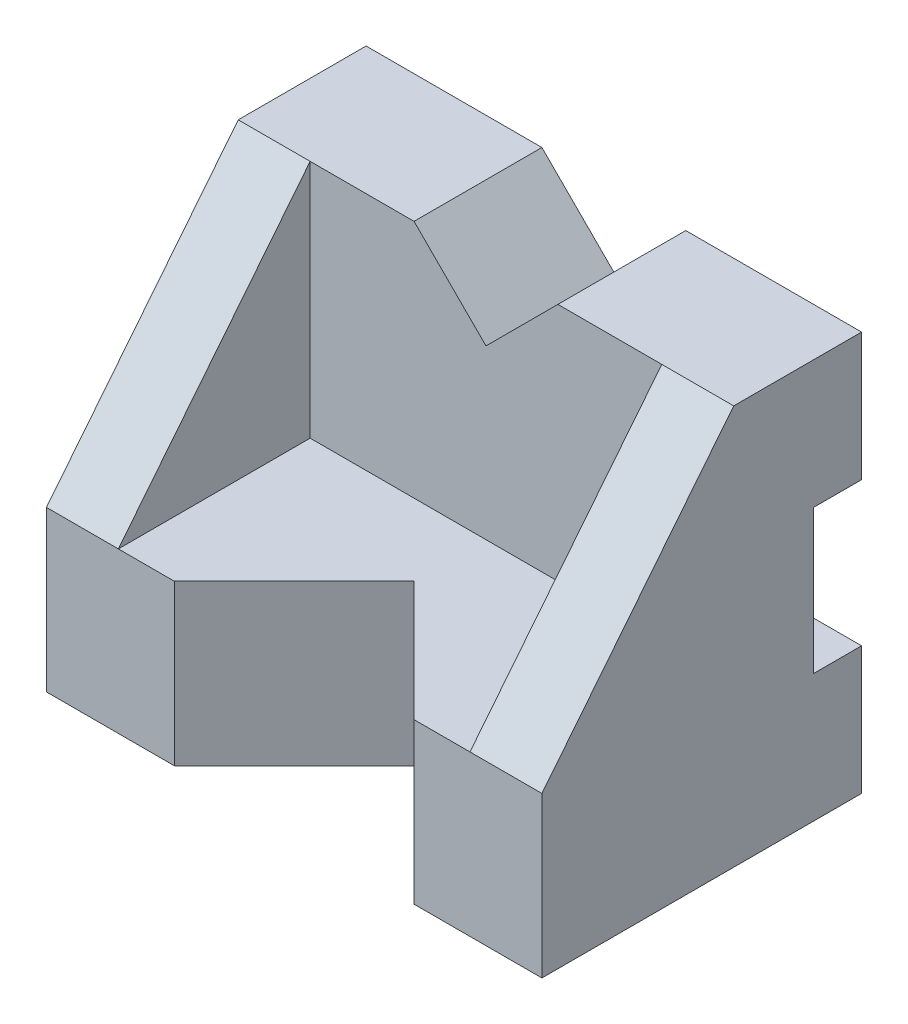
ISO-10303-21;
HEADER;
FILE_DESCRIPTION(('STEP AP214'),'2;1');
FILE_NAME('part.step','',(''),(''),'','','');
FILE_SCHEMA(('AUTOMOTIVE_DESIGN { 1 0 10303 214 1 1 1 1 }'));
ENDSEC;
DATA;
#1=APPLICATION_CONTEXT('core data for automotive mechanical design processes');
#2=APPLICATION_PROTOCOL_DEFINITION('international standard','automotive_design',2000,#1);
#3=PRODUCT_CONTEXT('',#1,'mechanical');
#4=PRODUCT('Part','Part','',(#3));
#5=PRODUCT_RELATED_PRODUCT_CATEGORY('part','',(#4));
#6=PRODUCT_DEFINITION_FORMATION('','',#4);
#7=PRODUCT_DEFINITION_CONTEXT('part definition',#1,'design');
#8=PRODUCT_DEFINITION('design','',#6,#7);
#9=PRODUCT_DEFINITION_SHAPE('','',#8);
#10=(LENGTH_UNIT() NAMED_UNIT(*) SI_UNIT(.MILLI.,.METRE.));
#11=(NAMED_UNIT(*) PLANE_ANGLE_UNIT() SI_UNIT($,.RADIAN.));
#12=(NAMED_UNIT(*) SI_UNIT($,.STERADIAN.) SOLID_ANGLE_UNIT());
#13=UNCERTAINTY_MEASURE_WITH_UNIT(LENGTH_MEASURE(1.E-05),#10,'distance_accuracy_value','');
#14=(GEOMETRIC_REPRESENTATION_CONTEXT(3) GLOBAL_UNCERTAINTY_ASSIGNED_CONTEXT((#13)) GLOBAL_UNIT_ASSIGNED_CONTEXT((#10,
#11,#12)) REPRESENTATION_CONTEXT('',''));
#15=CARTESIAN_POINT('',(0.,0.,0.));
#16=DIRECTION('',(0.,0.,1.));
#17=DIRECTION('',(1.,0.,0.));
#18=AXIS2_PLACEMENT_3D('',#15,#16,#17);
#19=CARTESIAN_POINT('',(0.,0.,32.));
#20=DIRECTION('',(0.,0.,1.));
#21=DIRECTION('',(1.,0.,0.));
#22=AXIS2_PLACEMENT_3D('',#19,#20,#21);
#23=PLANE('',#22);
#24=DIRECTION('',(0.707106781186547,0.707106781186548,0.));
#25=VECTOR('',#24,1.);
#26=CARTESIAN_POINT('',(40.,-40.,32.));
#27=LINE('',#26,#25);
#28=CARTESIAN_POINT('',(62.,-18.,32.));
#29=VERTEX_POINT('',#28);
#30=CARTESIAN_POINT('',(80.,0.,32.));
#31=VERTEX_POINT('',#30);
#32=EDGE_CURVE('E58',#29,#31,#27,.T.);
#33=ORIENTED_EDGE('',*,*,#32,.F.);
#34=DIRECTION('',(-0.707106781186548,0.707106781186547,0.));
#35=VECTOR('',#34,1.);
#36=CARTESIAN_POINT('',(22.,22.,32.));
#37=LINE('',#36,#35);
#38=CARTESIAN_POINT('',(44.,0.,32.));
#39=VERTEX_POINT('',#38);
#40=EDGE_CURVE('E176',#29,#39,#37,.T.);
#41=ORIENTED_EDGE('',*,*,#40,.T.);
#42=DIRECTION('',(-1.,0.,0.));
#43=VECTOR('',#42,1.);
#44=CARTESIAN_POINT('',(124.,0.,32.));
#45=LINE('',#44,#43);
#46=CARTESIAN_POINT('',(18.,0.,32.));
#47=VERTEX_POINT('',#46);
#48=EDGE_CURVE('E282',#39,#47,#45,.T.);
#49=ORIENTED_EDGE('',*,*,#48,.T.);
#50=DIRECTION('',(0.,-1.,0.));
#51=VECTOR('',#50,1.);
#52=CARTESIAN_POINT('',(18.,0.,32.));
#53=LINE('',#52,#51);
#54=CARTESIAN_POINT('',(18.,-60.,32.));
#55=VERTEX_POINT('',#54);
#56=EDGE_CURVE('E211',#47,#55,#53,.T.);
#57=ORIENTED_EDGE('',*,*,#56,.T.);
#58=DIRECTION('',(1.,0.,0.));
#59=VECTOR('',#58,1.);
#60=CARTESIAN_POINT('',(124.,-60.,32.));
#61=LINE('',#60,#59);
#62=CARTESIAN_POINT('',(106.,-60.,32.));
#63=VERTEX_POINT('',#62);
#64=EDGE_CURVE('E232',#55,#63,#61,.T.);
#65=ORIENTED_EDGE('',*,*,#64,.T.);
#66=DIRECTION('',(0.,1.,0.));
#67=VECTOR('',#66,1.);
#68=CARTESIAN_POINT('',(106.,0.,32.));
#69=LINE('',#68,#67);
#70=CARTESIAN_POINT('',(106.,0.,32.));
#71=VERTEX_POINT('',#70);
#72=EDGE_CURVE('E226',#63,#71,#69,.T.);
#73=ORIENTED_EDGE('',*,*,#72,.T.);
#74=EDGE_CURVE('E184',#71,#31,#45,.T.);
#75=ORIENTED_EDGE('',*,*,#74,.T.);
#76=EDGE_LOOP('',(#33,#41,#49,#57,#65,#73,#75));
#77=FACE_BOUND('',#76,.T.);
#78=ADVANCED_FACE('F44',(#77),#23,.T.);
#79=CARTESIAN_POINT('',(0.,0.,0.));
#80=DIRECTION('',(0.,0.,1.));
#81=DIRECTION('',(1.,0.,0.));
#82=AXIS2_PLACEMENT_3D('',#79,#80,#81);
#83=PLANE('',#82);
#84=DIRECTION('',(-0.707106781186548,0.707106781186547,0.));
#85=VECTOR('',#84,1.);
#86=CARTESIAN_POINT('',(22.,22.,0.));
#87=LINE('',#86,#85);
#88=CARTESIAN_POINT('',(62.,-18.,0.));
#89=VERTEX_POINT('',#88);
#90=CARTESIAN_POINT('',(44.,0.,0.));
#91=VERTEX_POINT('',#90);
#92=EDGE_CURVE('E186',#89,#91,#87,.T.);
#93=ORIENTED_EDGE('',*,*,#92,.F.);
#94=DIRECTION('',(0.707106781186547,0.707106781186548,0.));
#95=VECTOR('',#94,1.);
#96=CARTESIAN_POINT('',(40.,-40.,0.));
#97=LINE('',#96,#95);
#98=CARTESIAN_POINT('',(80.,0.,0.));
#99=VERTEX_POINT('',#98);
#100=EDGE_CURVE('E171',#89,#99,#97,.T.);
#101=ORIENTED_EDGE('',*,*,#100,.T.);
#102=DIRECTION('',(-1.,0.,0.));
#103=VECTOR('',#102,1.);
#104=CARTESIAN_POINT('',(124.,0.,0.));
#105=LINE('',#104,#103);
#106=CARTESIAN_POINT('',(124.,0.,0.));
#107=VERTEX_POINT('',#106);
#108=EDGE_CURVE('E285',#107,#99,#105,.T.);
#109=ORIENTED_EDGE('',*,*,#108,.F.);
#110=DIRECTION('',(0.,1.,0.));
#111=VECTOR('',#110,1.);
#112=CARTESIAN_POINT('',(124.,-100.,0.));
#113=LINE('',#112,#111);
#114=CARTESIAN_POINT('',(124.,-32.,0.));
#115=VERTEX_POINT('',#114);
#116=EDGE_CURVE('E293',#115,#107,#113,.T.);
#117=ORIENTED_EDGE('',*,*,#116,.F.);
#118=DIRECTION('',(-1.,0.,0.));
#119=VECTOR('',#118,1.);
#120=CARTESIAN_POINT('',(124.,-32.,0.));
#121=LINE('',#120,#119);
#122=CARTESIAN_POINT('',(0.,-32.,0.));
#123=VERTEX_POINT('',#122);
#124=EDGE_CURVE('E268',#115,#123,#121,.T.);
#125=ORIENTED_EDGE('',*,*,#124,.T.);
#126=DIRECTION('',(0.,-1.,0.));
#127=VECTOR('',#126,1.);
#128=CARTESIAN_POINT('',(0.,0.,0.));
#129=LINE('',#128,#127);
#130=CARTESIAN_POINT('',(0.,0.,0.));
#131=VERTEX_POINT('',#130);
#132=EDGE_CURVE('E289',#131,#123,#129,.T.);
#133=ORIENTED_EDGE('',*,*,#132,.F.);
#134=EDGE_CURVE('E275',#91,#131,#105,.T.);
#135=ORIENTED_EDGE('',*,*,#134,.F.);
#136=EDGE_LOOP('',(#93,#101,#109,#117,#125,#133,#135));
#137=FACE_BOUND('',#136,.T.);
#138=ADVANCED_FACE('F307',(#137),#83,.F.);
#139=CARTESIAN_POINT('',(124.,0.,32.));
#140=DIRECTION('',(0.,-1.,0.));
#141=DIRECTION('',(0.,0.,-1.));
#142=AXIS2_PLACEMENT_3D('',#139,#140,#141);
#143=PLANE('',#142);
#144=DIRECTION('',(0.,0.,1.));
#145=VECTOR('',#144,1.);
#146=CARTESIAN_POINT('',(44.,0.,32.));
#147=LINE('',#146,#145);
#148=EDGE_CURVE('E11',#91,#39,#147,.T.);
#149=ORIENTED_EDGE('',*,*,#148,.F.);
#150=ORIENTED_EDGE('',*,*,#134,.T.);
#151=DIRECTION('',(0.,0.,-1.));
#152=VECTOR('',#151,1.);
#153=CARTESIAN_POINT('',(0.,0.,32.));
#154=LINE('',#153,#152);
#155=CARTESIAN_POINT('',(0.,0.,32.));
#156=VERTEX_POINT('',#155);
#157=EDGE_CURVE('E303',#156,#131,#154,.T.);
#158=ORIENTED_EDGE('',*,*,#157,.F.);
#159=DIRECTION('',(-1.,0.,0.));
#160=VECTOR('',#159,1.);
#161=CARTESIAN_POINT('',(18.,0.,32.));
#162=LINE('',#161,#160);
#163=EDGE_CURVE('E218',#47,#156,#162,.T.);
#164=ORIENTED_EDGE('',*,*,#163,.F.);
#165=ORIENTED_EDGE('',*,*,#48,.F.);
#166=EDGE_LOOP('',(#149,#150,#158,#164,#165));
#167=FACE_BOUND('',#166,.T.);
#168=ADVANCED_FACE('F313',(#167),#143,.F.);
#169=CARTESIAN_POINT('',(0.,-60.,80.));
#170=DIRECTION('',(0.,0.,1.));
#171=DIRECTION('',(1.,0.,0.));
#172=AXIS2_PLACEMENT_3D('',#169,#170,#171);
#173=PLANE('',#172);
#174=DIRECTION('',(0.,1.,0.));
#175=VECTOR('',#174,1.);
#176=CARTESIAN_POINT('',(32.,-100.,80.));
#177=LINE('',#176,#175);
#178=CARTESIAN_POINT('',(32.,-100.,80.));
#179=VERTEX_POINT('',#178);
#180=CARTESIAN_POINT('',(32.,-60.,80.));
#181=VERTEX_POINT('',#180);
#182=EDGE_CURVE('E204',#179,#181,#177,.T.);
#183=ORIENTED_EDGE('',*,*,#182,.T.);
#184=DIRECTION('',(-1.,0.,0.));
#185=VECTOR('',#184,1.);
#186=CARTESIAN_POINT('',(0.,-60.,80.));
#187=LINE('',#186,#185);
#188=CARTESIAN_POINT('',(18.,-60.,80.));
#189=VERTEX_POINT('',#188);
#190=EDGE_CURVE('E240',#181,#189,#187,.T.);
#191=ORIENTED_EDGE('',*,*,#190,.T.);
#192=DIRECTION('',(-1.,0.,0.));
#193=VECTOR('',#192,1.);
#194=CARTESIAN_POINT('',(18.,-60.,80.));
#195=LINE('',#194,#193);
#196=CARTESIAN_POINT('',(0.,-60.,80.));
#197=VERTEX_POINT('',#196);
#198=EDGE_CURVE('E220',#189,#197,#195,.T.);
#199=ORIENTED_EDGE('',*,*,#198,.T.);
#200=DIRECTION('',(0.,-1.,0.));
#201=VECTOR('',#200,1.);
#202=CARTESIAN_POINT('',(0.,-60.,80.));
#203=LINE('',#202,#201);
#204=CARTESIAN_POINT('',(0.,-100.,80.));
#205=VERTEX_POINT('',#204);
#206=EDGE_CURVE('E246',#197,#205,#203,.T.);
#207=ORIENTED_EDGE('',*,*,#206,.T.);
#208=DIRECTION('',(-1.,0.,0.));
#209=VECTOR('',#208,1.);
#210=CARTESIAN_POINT('',(0.,-100.,80.));
#211=LINE('',#210,#209);
#212=EDGE_CURVE('E231',#179,#205,#211,.T.);
#213=ORIENTED_EDGE('',*,*,#212,.F.);
#214=EDGE_LOOP('',(#183,#191,#199,#207,#213));
#215=FACE_BOUND('',#214,.T.);
#216=ADVANCED_FACE('F358',(#215),#173,.T.);
#217=CARTESIAN_POINT('',(0.,-60.,0.));
#218=DIRECTION('',(0.,1.,0.));
#219=DIRECTION('',(0.,0.,1.));
#220=AXIS2_PLACEMENT_3D('',#217,#218,#219);
#221=PLANE('',#220);
#222=DIRECTION('',(-0.707106781186548,0.,0.707106781186548));
#223=VECTOR('',#222,1.);
#224=CARTESIAN_POINT('',(56.,-60.,56.));
#225=LINE('',#224,#223);
#226=CARTESIAN_POINT('',(62.,-60.,50.));
#227=VERTEX_POINT('',#226);
#228=EDGE_CURVE('E191',#227,#181,#225,.T.);
#229=ORIENTED_EDGE('',*,*,#228,.F.);
#230=DIRECTION('',(-0.707106781186548,0.,-0.707106781186548));
#231=VECTOR('',#230,1.);
#232=CARTESIAN_POINT('',(6.,-60.,-6.));
#233=LINE('',#232,#231);
#234=CARTESIAN_POINT('',(92.,-60.,80.));
#235=VERTEX_POINT('',#234);
#236=EDGE_CURVE('E192',#235,#227,#233,.T.);
#237=ORIENTED_EDGE('',*,*,#236,.F.);
#238=CARTESIAN_POINT('',(106.,-60.,80.));
#239=VERTEX_POINT('',#238);
#240=EDGE_CURVE('E243',#239,#235,#187,.T.);
#241=ORIENTED_EDGE('',*,*,#240,.F.);
#242=DIRECTION('',(0.,0.,-1.));
#243=VECTOR('',#242,1.);
#244=CARTESIAN_POINT('',(106.,-60.,32.));
#245=LINE('',#244,#243);
#246=EDGE_CURVE('E222',#239,#63,#245,.T.);
#247=ORIENTED_EDGE('',*,*,#246,.T.);
#248=ORIENTED_EDGE('',*,*,#64,.F.);
#249=DIRECTION('',(0.,0.,1.));
#250=VECTOR('',#249,1.);
#251=CARTESIAN_POINT('',(18.,-60.,32.));
#252=LINE('',#251,#250);
#253=EDGE_CURVE('E206',#55,#189,#252,.T.);
#254=ORIENTED_EDGE('',*,*,#253,.T.);
#255=ORIENTED_EDGE('',*,*,#190,.F.);
#256=EDGE_LOOP('',(#229,#237,#241,#247,#248,#254,#255));
#257=FACE_BOUND('',#256,.T.);
#258=ADVANCED_FACE('F329',(#257),#221,.T.);
#259=ORIENTED_EDGE('',*,*,#108,.T.);
#260=DIRECTION('',(0.,0.,1.));
#261=VECTOR('',#260,1.);
#262=CARTESIAN_POINT('',(80.,0.,32.));
#263=LINE('',#262,#261);
#264=EDGE_CURVE('E52',#99,#31,#263,.T.);
#265=ORIENTED_EDGE('',*,*,#264,.T.);
#266=ORIENTED_EDGE('',*,*,#74,.F.);
#267=CARTESIAN_POINT('',(124.,0.,32.));
#268=VERTEX_POINT('',#267);
#269=EDGE_CURVE('E279',#268,#71,#45,.T.);
#270=ORIENTED_EDGE('',*,*,#269,.F.);
#271=DIRECTION('',(0.,0.,-1.));
#272=VECTOR('',#271,1.);
#273=CARTESIAN_POINT('',(124.,0.,32.));
#274=LINE('',#273,#272);
#275=EDGE_CURVE('E278',#268,#107,#274,.T.);
#276=ORIENTED_EDGE('',*,*,#275,.T.);
#277=EDGE_LOOP('',(#259,#265,#266,#270,#276));
#278=FACE_BOUND('',#277,.T.);
#279=ADVANCED_FACE('F50',(#278),#143,.F.);
#280=CARTESIAN_POINT('',(0.,0.,32.));
#281=DIRECTION('',(1.,0.,0.));
#282=DIRECTION('',(0.,0.,-1.));
#283=AXIS2_PLACEMENT_3D('',#280,#281,#282);
#284=PLANE('',#283);
#285=ORIENTED_EDGE('',*,*,#132,.T.);
#286=DIRECTION('',(0.,0.,-1.));
#287=VECTOR('',#286,1.);
#288=CARTESIAN_POINT('',(0.,-32.,12.));
#289=LINE('',#288,#287);
#290=CARTESIAN_POINT('',(0.,-32.,12.));
#291=VERTEX_POINT('',#290);
#292=EDGE_CURVE('E257',#291,#123,#289,.T.);
#293=ORIENTED_EDGE('',*,*,#292,.F.);
#294=DIRECTION('',(0.,1.,0.));
#295=VECTOR('',#294,1.);
#296=CARTESIAN_POINT('',(0.,-68.,12.));
#297=LINE('',#296,#295);
#298=CARTESIAN_POINT('',(0.,-68.,12.));
#299=VERTEX_POINT('',#298);
#300=EDGE_CURVE('E263',#299,#291,#297,.T.);
#301=ORIENTED_EDGE('',*,*,#300,.F.);
#302=DIRECTION('',(0.,0.,1.));
#303=VECTOR('',#302,1.);
#304=CARTESIAN_POINT('',(0.,-68.,0.));
#305=LINE('',#304,#303);
#306=CARTESIAN_POINT('',(0.,-68.,0.));
#307=VERTEX_POINT('',#306);
#308=EDGE_CURVE('E248',#307,#299,#305,.T.);
#309=ORIENTED_EDGE('',*,*,#308,.F.);
#310=CARTESIAN_POINT('',(0.,-100.,0.));
#311=VERTEX_POINT('',#310);
#312=EDGE_CURVE('E283',#307,#311,#129,.T.);
#313=ORIENTED_EDGE('',*,*,#312,.T.);
#314=DIRECTION('',(0.,0.,-1.));
#315=VECTOR('',#314,1.);
#316=CARTESIAN_POINT('',(0.,-100.,32.));
#317=LINE('',#316,#315);
#318=EDGE_CURVE('E297',#205,#311,#317,.T.);
#319=ORIENTED_EDGE('',*,*,#318,.F.);
#320=ORIENTED_EDGE('',*,*,#206,.F.);
#321=DIRECTION('',(0.,0.78086880944303,-0.624695047554424));
#322=VECTOR('',#321,1.);
#323=CARTESIAN_POINT('',(0.,-60.,80.));
#324=LINE('',#323,#322);
#325=EDGE_CURVE('E203',#197,#156,#324,.T.);
#326=ORIENTED_EDGE('',*,*,#325,.T.);
#327=ORIENTED_EDGE('',*,*,#157,.T.);
#328=EDGE_LOOP('',(#285,#293,#301,#309,#313,#319,#320,#326,#327));
#329=FACE_BOUND('',#328,.T.);
#330=ADVANCED_FACE('F354',(#329),#284,.F.);
#331=CARTESIAN_POINT('',(0.,-100.,32.));
#332=DIRECTION('',(0.,1.,0.));
#333=DIRECTION('',(0.,0.,1.));
#334=AXIS2_PLACEMENT_3D('',#331,#332,#333);
#335=PLANE('',#334);
#336=DIRECTION('',(-0.707106781186548,0.,-0.707106781186548));
#337=VECTOR('',#336,1.);
#338=CARTESIAN_POINT('',(6.,-100.,-6.));
#339=LINE('',#338,#337);
#340=CARTESIAN_POINT('',(92.,-100.,80.));
#341=VERTEX_POINT('',#340);
#342=CARTESIAN_POINT('',(62.,-100.,50.));
#343=VERTEX_POINT('',#342);
#344=EDGE_CURVE('E69',#341,#343,#339,.T.);
#345=ORIENTED_EDGE('',*,*,#344,.T.);
#346=DIRECTION('',(-0.707106781186548,0.,0.707106781186548));
#347=VECTOR('',#346,1.);
#348=CARTESIAN_POINT('',(56.,-100.,56.));
#349=LINE('',#348,#347);
#350=EDGE_CURVE('E194',#343,#179,#349,.T.);
#351=ORIENTED_EDGE('',*,*,#350,.T.);
#352=ORIENTED_EDGE('',*,*,#212,.T.);
#353=ORIENTED_EDGE('',*,*,#318,.T.);
#354=DIRECTION('',(1.,0.,0.));
#355=VECTOR('',#354,1.);
#356=CARTESIAN_POINT('',(0.,-100.,0.));
#357=LINE('',#356,#355);
#358=CARTESIAN_POINT('',(124.,-100.,0.));
#359=VERTEX_POINT('',#358);
#360=EDGE_CURVE('E288',#311,#359,#357,.T.);
#361=ORIENTED_EDGE('',*,*,#360,.T.);
#362=DIRECTION('',(0.,0.,-1.));
#363=VECTOR('',#362,1.);
#364=CARTESIAN_POINT('',(124.,-100.,32.));
#365=LINE('',#364,#363);
#366=CARTESIAN_POINT('',(124.,-100.,80.));
#367=VERTEX_POINT('',#366);
#368=EDGE_CURVE('E300',#367,#359,#365,.T.);
#369=ORIENTED_EDGE('',*,*,#368,.F.);
#370=EDGE_CURVE('E238',#367,#341,#211,.T.);
#371=ORIENTED_EDGE('',*,*,#370,.T.);
#372=EDGE_LOOP('',(#345,#351,#352,#353,#361,#369,#371));
#373=FACE_BOUND('',#372,.T.);
#374=ADVANCED_FACE('F365',(#373),#335,.F.);
#375=CARTESIAN_POINT('',(124.,-100.,32.));
#376=DIRECTION('',(-1.,0.,0.));
#377=DIRECTION('',(0.,0.,1.));
#378=AXIS2_PLACEMENT_3D('',#375,#376,#377);
#379=PLANE('',#378);
#380=ORIENTED_EDGE('',*,*,#275,.F.);
#381=DIRECTION('',(0.,-0.78086880944303,0.624695047554424));
#382=VECTOR('',#381,1.);
#383=CARTESIAN_POINT('',(124.,-60.,80.));
#384=LINE('',#383,#382);
#385=CARTESIAN_POINT('',(124.,-60.,80.));
#386=VERTEX_POINT('',#385);
#387=EDGE_CURVE('E221',#268,#386,#384,.T.);
#388=ORIENTED_EDGE('',*,*,#387,.T.);
#389=DIRECTION('',(0.,-1.,0.));
#390=VECTOR('',#389,1.);
#391=CARTESIAN_POINT('',(124.,-60.,80.));
#392=LINE('',#391,#390);
#393=EDGE_CURVE('E245',#386,#367,#392,.T.);
#394=ORIENTED_EDGE('',*,*,#393,.T.);
#395=ORIENTED_EDGE('',*,*,#368,.T.);
#396=CARTESIAN_POINT('',(124.,-68.,0.));
#397=VERTEX_POINT('',#396);
#398=EDGE_CURVE('E292',#359,#397,#113,.T.);
#399=ORIENTED_EDGE('',*,*,#398,.T.);
#400=DIRECTION('',(0.,0.,1.));
#401=VECTOR('',#400,1.);
#402=CARTESIAN_POINT('',(124.,-68.,0.));
#403=LINE('',#402,#401);
#404=CARTESIAN_POINT('',(124.,-68.,12.));
#405=VERTEX_POINT('',#404);
#406=EDGE_CURVE('E255',#397,#405,#403,.T.);
#407=ORIENTED_EDGE('',*,*,#406,.T.);
#408=DIRECTION('',(0.,1.,0.));
#409=VECTOR('',#408,1.);
#410=CARTESIAN_POINT('',(124.,-68.,12.));
#411=LINE('',#410,#409);
#412=CARTESIAN_POINT('',(124.,-32.,12.));
#413=VERTEX_POINT('',#412);
#414=EDGE_CURVE('E253',#405,#413,#411,.T.);
#415=ORIENTED_EDGE('',*,*,#414,.T.);
#416=DIRECTION('',(0.,0.,-1.));
#417=VECTOR('',#416,1.);
#418=CARTESIAN_POINT('',(124.,-32.,12.));
#419=LINE('',#418,#417);
#420=EDGE_CURVE('E256',#413,#115,#419,.T.);
#421=ORIENTED_EDGE('',*,*,#420,.T.);
#422=ORIENTED_EDGE('',*,*,#116,.T.);
#423=EDGE_LOOP('',(#380,#388,#394,#395,#399,#407,#415,#421,#422));
#424=FACE_BOUND('',#423,.T.);
#425=ADVANCED_FACE('F343',(#424),#379,.F.);
#426=ORIENTED_EDGE('',*,*,#312,.F.);
#427=DIRECTION('',(-1.,0.,0.));
#428=VECTOR('',#427,1.);
#429=CARTESIAN_POINT('',(124.,-68.,0.));
#430=LINE('',#429,#428);
#431=EDGE_CURVE('E265',#397,#307,#430,.T.);
#432=ORIENTED_EDGE('',*,*,#431,.F.);
#433=ORIENTED_EDGE('',*,*,#398,.F.);
#434=ORIENTED_EDGE('',*,*,#360,.F.);
#435=EDGE_LOOP('',(#426,#432,#433,#434));
#436=FACE_BOUND('',#435,.T.);
#437=ADVANCED_FACE('F366',(#436),#83,.F.);
#438=CARTESIAN_POINT('',(124.,-32.,12.));
#439=DIRECTION('',(0.,1.,0.));
#440=DIRECTION('',(0.,0.,1.));
#441=AXIS2_PLACEMENT_3D('',#438,#439,#440);
#442=PLANE('',#441);
#443=ORIENTED_EDGE('',*,*,#292,.T.);
#444=ORIENTED_EDGE('',*,*,#124,.F.);
#445=ORIENTED_EDGE('',*,*,#420,.F.);
#446=DIRECTION('',(-1.,0.,0.));
#447=VECTOR('',#446,1.);
#448=CARTESIAN_POINT('',(124.,-32.,12.));
#449=LINE('',#448,#447);
#450=EDGE_CURVE('E271',#413,#291,#449,.T.);
#451=ORIENTED_EDGE('',*,*,#450,.T.);
#452=EDGE_LOOP('',(#443,#444,#445,#451));
#453=FACE_BOUND('',#452,.T.);
#454=ADVANCED_FACE('F372',(#453),#442,.F.);
#455=CARTESIAN_POINT('',(124.,-68.,12.));
#456=DIRECTION('',(0.,0.,1.));
#457=DIRECTION('',(1.,0.,0.));
#458=AXIS2_PLACEMENT_3D('',#455,#456,#457);
#459=PLANE('',#458);
#460=ORIENTED_EDGE('',*,*,#300,.T.);
#461=ORIENTED_EDGE('',*,*,#450,.F.);
#462=ORIENTED_EDGE('',*,*,#414,.F.);
#463=DIRECTION('',(-1.,0.,0.));
#464=VECTOR('',#463,1.);
#465=CARTESIAN_POINT('',(124.,-68.,12.));
#466=LINE('',#465,#464);
#467=EDGE_CURVE('E273',#405,#299,#466,.T.);
#468=ORIENTED_EDGE('',*,*,#467,.T.);
#469=EDGE_LOOP('',(#460,#461,#462,#468));
#470=FACE_BOUND('',#469,.T.);
#471=ADVANCED_FACE('F373',(#470),#459,.F.);
#472=CARTESIAN_POINT('',(124.,-68.,0.));
#473=DIRECTION('',(0.,-1.,0.));
#474=DIRECTION('',(0.,0.,-1.));
#475=AXIS2_PLACEMENT_3D('',#472,#473,#474);
#476=PLANE('',#475);
#477=ORIENTED_EDGE('',*,*,#308,.T.);
#478=ORIENTED_EDGE('',*,*,#467,.F.);
#479=ORIENTED_EDGE('',*,*,#406,.F.);
#480=ORIENTED_EDGE('',*,*,#431,.T.);
#481=EDGE_LOOP('',(#477,#478,#479,#480));
#482=FACE_BOUND('',#481,.T.);
#483=ADVANCED_FACE('F369',(#482),#476,.F.);
#484=DIRECTION('',(0.,1.,0.));
#485=VECTOR('',#484,1.);
#486=CARTESIAN_POINT('',(92.,-100.,80.));
#487=LINE('',#486,#485);
#488=EDGE_CURVE('E200',#341,#235,#487,.T.);
#489=ORIENTED_EDGE('',*,*,#488,.F.);
#490=ORIENTED_EDGE('',*,*,#370,.F.);
#491=ORIENTED_EDGE('',*,*,#393,.F.);
#492=EDGE_CURVE('E237',#386,#239,#187,.T.);
#493=ORIENTED_EDGE('',*,*,#492,.T.);
#494=ORIENTED_EDGE('',*,*,#240,.T.);
#495=EDGE_LOOP('',(#489,#490,#491,#493,#494));
#496=FACE_BOUND('',#495,.T.);
#497=ADVANCED_FACE('F342',(#496),#173,.T.);
#498=CARTESIAN_POINT('',(106.,-60.,80.));
#499=DIRECTION('',(0.,0.624695047554424,0.78086880944303));
#500=DIRECTION('',(0.,-0.78086880944303,0.624695047554424));
#501=AXIS2_PLACEMENT_3D('',#498,#499,#500);
#502=PLANE('',#501);
#503=ORIENTED_EDGE('',*,*,#387,.F.);
#504=ORIENTED_EDGE('',*,*,#269,.T.);
#505=DIRECTION('',(0.,-0.78086880944303,0.624695047554424));
#506=VECTOR('',#505,1.);
#507=CARTESIAN_POINT('',(106.,-60.,80.));
#508=LINE('',#507,#506);
#509=EDGE_CURVE('E229',#71,#239,#508,.T.);
#510=ORIENTED_EDGE('',*,*,#509,.T.);
#511=ORIENTED_EDGE('',*,*,#492,.F.);
#512=EDGE_LOOP('',(#503,#504,#510,#511));
#513=FACE_BOUND('',#512,.T.);
#514=ADVANCED_FACE('F337',(#513),#502,.T.);
#515=CARTESIAN_POINT('',(106.,0.,0.));
#516=DIRECTION('',(1.,0.,0.));
#517=DIRECTION('',(0.,0.,-1.));
#518=AXIS2_PLACEMENT_3D('',#515,#516,#517);
#519=PLANE('',#518);
#520=ORIENTED_EDGE('',*,*,#246,.F.);
#521=ORIENTED_EDGE('',*,*,#509,.F.);
#522=ORIENTED_EDGE('',*,*,#72,.F.);
#523=EDGE_LOOP('',(#520,#521,#522));
#524=FACE_BOUND('',#523,.T.);
#525=ADVANCED_FACE('F335',(#524),#519,.F.);
#526=CARTESIAN_POINT('',(18.,-60.,80.));
#527=DIRECTION('',(0.,0.624695047554424,0.78086880944303));
#528=DIRECTION('',(0.,-0.78086880944303,0.624695047554424));
#529=AXIS2_PLACEMENT_3D('',#526,#527,#528);
#530=PLANE('',#529);
#531=ORIENTED_EDGE('',*,*,#325,.F.);
#532=ORIENTED_EDGE('',*,*,#198,.F.);
#533=DIRECTION('',(0.,0.78086880944303,-0.624695047554424));
#534=VECTOR('',#533,1.);
#535=CARTESIAN_POINT('',(18.,-60.,80.));
#536=LINE('',#535,#534);
#537=EDGE_CURVE('E212',#189,#47,#536,.T.);
#538=ORIENTED_EDGE('',*,*,#537,.T.);
#539=ORIENTED_EDGE('',*,*,#163,.T.);
#540=EDGE_LOOP('',(#531,#532,#538,#539));
#541=FACE_BOUND('',#540,.T.);
#542=ADVANCED_FACE('F325',(#541),#530,.T.);
#543=CARTESIAN_POINT('',(18.,0.,0.));
#544=DIRECTION('',(1.,0.,0.));
#545=DIRECTION('',(0.,0.,-1.));
#546=AXIS2_PLACEMENT_3D('',#543,#544,#545);
#547=PLANE('',#546);
#548=ORIENTED_EDGE('',*,*,#253,.F.);
#549=ORIENTED_EDGE('',*,*,#56,.F.);
#550=ORIENTED_EDGE('',*,*,#537,.F.);
#551=EDGE_LOOP('',(#548,#549,#550));
#552=FACE_BOUND('',#551,.T.);
#553=ADVANCED_FACE('F321',(#552),#547,.T.);
#554=CARTESIAN_POINT('',(56.,-100.,56.));
#555=DIRECTION('',(-0.707106781186548,0.,-0.707106781186548));
#556=DIRECTION('',(-0.707106781186548,0.,0.707106781186548));
#557=AXIS2_PLACEMENT_3D('',#554,#555,#556);
#558=PLANE('',#557);
#559=ORIENTED_EDGE('',*,*,#228,.T.);
#560=ORIENTED_EDGE('',*,*,#182,.F.);
#561=ORIENTED_EDGE('',*,*,#350,.F.);
#562=DIRECTION('',(0.,1.,0.));
#563=VECTOR('',#562,1.);
#564=CARTESIAN_POINT('',(62.,-100.,50.));
#565=LINE('',#564,#563);
#566=EDGE_CURVE('E202',#343,#227,#565,.T.);
#567=ORIENTED_EDGE('',*,*,#566,.T.);
#568=EDGE_LOOP('',(#559,#560,#561,#567));
#569=FACE_BOUND('',#568,.T.);
#570=ADVANCED_FACE('F359',(#569),#558,.F.);
#571=CARTESIAN_POINT('',(6.,-100.,-6.));
#572=DIRECTION('',(0.707106781186548,0.,-0.707106781186548));
#573=DIRECTION('',(-0.707106781186548,0.,-0.707106781186548));
#574=AXIS2_PLACEMENT_3D('',#571,#572,#573);
#575=PLANE('',#574);
#576=ORIENTED_EDGE('',*,*,#236,.T.);
#577=ORIENTED_EDGE('',*,*,#566,.F.);
#578=ORIENTED_EDGE('',*,*,#344,.F.);
#579=ORIENTED_EDGE('',*,*,#488,.T.);
#580=EDGE_LOOP('',(#576,#577,#578,#579));
#581=FACE_BOUND('',#580,.T.);
#582=ADVANCED_FACE('F436',(#581),#575,.F.);
#583=CARTESIAN_POINT('',(22.,22.,-8.));
#584=DIRECTION('',(0.707106781186547,0.707106781186548,0.));
#585=DIRECTION('',(-0.707106781186548,0.707106781186547,0.));
#586=AXIS2_PLACEMENT_3D('',#583,#584,#585);
#587=PLANE('',#586);
#588=ORIENTED_EDGE('',*,*,#92,.T.);
#589=ORIENTED_EDGE('',*,*,#148,.T.);
#590=ORIENTED_EDGE('',*,*,#40,.F.);
#591=DIRECTION('',(0.,0.,1.));
#592=VECTOR('',#591,1.);
#593=CARTESIAN_POINT('',(62.,-18.,-8.));
#594=LINE('',#593,#592);
#595=EDGE_CURVE('E170',#89,#29,#594,.T.);
#596=ORIENTED_EDGE('',*,*,#595,.F.);
#597=EDGE_LOOP('',(#588,#589,#590,#596));
#598=FACE_BOUND('',#597,.T.);
#599=ADVANCED_FACE('F180',(#598),#587,.T.);
#600=CARTESIAN_POINT('',(40.,-40.,-8.));
#601=DIRECTION('',(0.707106781186548,-0.707106781186547,0.));
#602=DIRECTION('',(0.707106781186547,0.707106781186548,0.));
#603=AXIS2_PLACEMENT_3D('',#600,#601,#602);
#604=PLANE('',#603);
#605=ORIENTED_EDGE('',*,*,#595,.T.);
#606=ORIENTED_EDGE('',*,*,#32,.T.);
#607=ORIENTED_EDGE('',*,*,#264,.F.);
#608=ORIENTED_EDGE('',*,*,#100,.F.);
#609=EDGE_LOOP('',(#605,#606,#607,#608));
#610=FACE_BOUND('',#609,.T.);
#611=ADVANCED_FACE('F169',(#610),#604,.F.);
#612=CLOSED_SHELL('',(#78,#138,#168,#216,#258,#279,#330,#374,#425,#437,#454,#471,#483,#497,#514,
#525,#542,#553,#570,#582,#599,#611));
#613=MANIFOLD_SOLID_BREP('B2',#612);
#614=ADVANCED_BREP_SHAPE_REPRESENTATION('',(#18,#613),#14);
#615=SHAPE_DEFINITION_REPRESENTATION(#9,#614);
ENDSEC;
END-ISO-10303-21;
